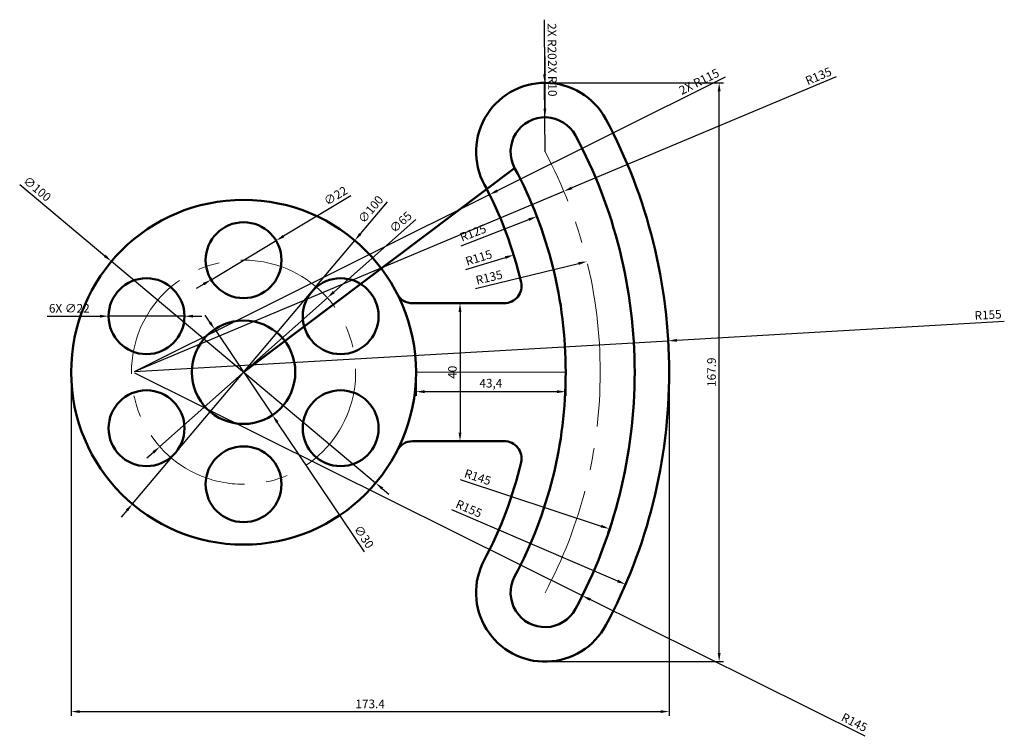
# Model space of a CAD drawing. Units: millimetres. Extents: x 3074 to 3359, y 1439 to 1647.
import ezdxf

# ---------------------------------------------------------------- set-up
doc = ezdxf.new("R2010")
doc.units = ezdxf.units.MM
doc.linetypes.add('CENTER', pattern=[50.8, 31.75, -6.35, 6.35, -6.35])
for name, color, linetype, lineweight in [('M-CNTR', 4, 'CENTER', 18), ('M-CONS', 8, 'Continuous', 13), ('M-DIMS', 2, 'Continuous', 25), ('M-OUTL', 7, 'Continuous', 50)]:
    doc.layers.add(name, color=color, linetype=linetype, lineweight=lineweight)
doc.styles.get("Standard").update_dxf_attribs({"font": 'arial.ttf'})
doc.dimstyles.new('ISO-25', dxfattribs={"dimtxt": 2.5, "dimasz": 2.5, "dimexe": 1.25, "dimexo": 0.625, "dimtad": 1, "dimtxsty": 'Standard', "dimcen": 2.5, "dimadec": 0, "dimazin": 0, "dimtfac": 1, "dimtmove": 0, "dimatfit": 3, "dimfxl": 1, "dimarcsym": 0})

# ---------------------------------------------------------------- blocks, each defined once
blk = doc.blocks.new('*D1')
at = {"layer": 'Defpoints', "color": 0, "transparency": 16777216}
for p in [(3188.62, 1545.09), (3232.02, 1545.09), (3188.62, 1539.45)]:
    blk.add_point(p, dxfattribs=at)
at = {"layer": 'M-DIMS', "color": 0, "lineweight": -2, "transparency": 16777216}
for p, q in [((3188.62, 1544.47), (3188.62, 1538.2)), ((3232.02, 1544.47), (3232.02, 1538.2)), ((3229.52, 1539.45), (3191.12, 1539.45))]:
    blk.add_line(p, q, dxfattribs=at)
at = {"layer": 'M-DIMS', "color": 0, "transparency": 16777216}
for points in [[(3191.12, 1539.87), (3191.12, 1539.03), (3188.62, 1539.45)], [(3229.52, 1539.87), (3229.52, 1539.03), (3232.02, 1539.45)]]:
    blk.add_solid(points, dxfattribs=at)
at = {"layer": 'M-DIMS', "color": 0, "transparency": 16777216, "insert": (3210.32, 1541.58), "char_height": 2.5, "attachment_point": 5}
blk.add_mtext('43,4', dxfattribs=at)
blk = doc.blocks.new('*D2')
at = {"layer": 'Defpoints', "color": 0, "transparency": 16777216}
for p in [(3223.66, 1590.27), (3107.02, 1545.32)]:
    blk.add_point(p, dxfattribs=at)
at = {"layer": 'M-DIMS', "color": 0, "lineweight": -2, "transparency": 16777216}
blk.add_line((3201.67, 1581.8), (3221.32, 1589.37), dxfattribs=at)
at = {"layer": 'M-DIMS', "color": 0, "transparency": 16777216}
blk.add_solid([(3221.17, 1589.76), (3221.47, 1588.98), (3223.66, 1590.27)], dxfattribs=at)
at = {"layer": 'M-DIMS', "color": 0, "transparency": 16777216, "insert": (3205.27, 1585.22), "char_height": 2.5, "attachment_point": 5, "rotation": 21.0776}
blk.add_mtext('R125', dxfattribs=at)
blk = doc.blocks.new('*D3')
at = {"layer": 'Defpoints', "color": 0, "transparency": 16777216}
for p in [(3216.94, 1579.11), (3107.02, 1545.32)]:
    blk.add_point(p, dxfattribs=at)
at = {"layer": 'M-DIMS', "color": 0, "lineweight": -2, "transparency": 16777216}
blk.add_line((3203.08, 1574.85), (3214.56, 1578.37), dxfattribs=at)
at = {"layer": 'M-DIMS', "color": 0, "transparency": 16777216}
blk.add_solid([(3214.43, 1578.77), (3214.68, 1577.97), (3216.94, 1579.11)], dxfattribs=at)
at = {"layer": 'M-DIMS', "color": 0, "transparency": 16777216, "insert": (3206.91, 1578.01), "char_height": 2.5, "attachment_point": 5, "rotation": 17.0867}
blk.add_mtext('R115', dxfattribs=at)
blk = doc.blocks.new('*D4')
at = {"layer": 'Defpoints', "color": 0, "transparency": 16777216}
for p in [(3238.2, 1577.23), (3107.02, 1545.32)]:
    blk.add_point(p, dxfattribs=at)
at = {"layer": 'M-DIMS', "color": 0, "lineweight": -2, "transparency": 16777216}
blk.add_line((3205.88, 1569.37), (3235.77, 1576.63), dxfattribs=at)
at = {"layer": 'M-DIMS', "color": 0, "transparency": 16777216}
blk.add_solid([(3235.67, 1577.04), (3235.87, 1576.23), (3238.2, 1577.23)], dxfattribs=at)
at = {"layer": 'M-DIMS', "color": 0, "transparency": 16777216, "insert": (3209.9, 1572.3), "char_height": 2.5, "attachment_point": 5, "rotation": 13.6714}
blk.add_mtext('R135', dxfattribs=at)
blk = doc.blocks.new('*D5')
at = {"layer": 'Defpoints', "color": 0, "transparency": 16777216}
for p in [(3107.02, 1545.32), (3244.65, 1499.68)]:
    blk.add_point(p, dxfattribs=at)
at = {"layer": 'M-DIMS', "color": 0, "lineweight": -2, "transparency": 16777216}
blk.add_line((3201.45, 1514), (3242.28, 1500.46), dxfattribs=at)
blk.add_arc((3107.02, 1545.32), 145, 341.1592, 359.6499, dxfattribs=at)
at = {"layer": 'M-DIMS', "color": 0, "transparency": 16777216}
blk.add_solid([(3242.41, 1500.86), (3242.15, 1500.07), (3244.65, 1499.68)], dxfattribs=at)
at = {"layer": 'M-DIMS', "color": 0, "transparency": 16777216, "insert": (3206.41, 1514.36), "char_height": 2.5, "attachment_point": 5, "rotation": 341.6531}
blk.add_mtext('R145', dxfattribs=at)
blk = doc.blocks.new('*D6')
at = {"layer": 'Defpoints', "color": 0, "transparency": 16777216}
for p in [(3107.02, 1544.87), (3249.38, 1483.55)]:
    blk.add_point(p, dxfattribs=at)
at = {"layer": 'M-DIMS', "color": 0, "lineweight": -2, "transparency": 16777216}
blk.add_line((3198.87, 1505.31), (3247.08, 1484.54), dxfattribs=at)
at = {"layer": 'M-DIMS', "color": 0, "transparency": 16777216}
blk.add_solid([(3247.24, 1484.92), (3246.91, 1484.15), (3249.38, 1483.55)], dxfattribs=at)
at = {"layer": 'M-DIMS', "color": 0, "transparency": 16777216, "insert": (3203.84, 1505.23), "char_height": 2.5, "attachment_point": 5, "rotation": 336.6959}
blk.add_mtext('R155', dxfattribs=at)
blk = doc.blocks.new('*D7')
at = {"layer": 'Defpoints', "color": 0, "transparency": 16777216}
for p in [(3170.86, 1583.31), (3106.38, 1506.87)]:
    blk.add_point(p, dxfattribs=at)
at = {"layer": 'M-DIMS', "color": 0, "lineweight": -2, "transparency": 16777216}
for p, q in [((3180.28, 1594.48), (3172.47, 1585.22)), ((3106.38, 1506.87), (3170.86, 1583.31)), ((3104.77, 1504.96), (3103.16, 1503.05))]:
    blk.add_line(p, q, dxfattribs=at)
at = {"layer": 'M-DIMS', "color": 0, "transparency": 16777216}
for points in [[(3172.15, 1585.49), (3172.79, 1584.96), (3170.86, 1583.31)], [(3104.45, 1505.23), (3105.09, 1504.69), (3106.38, 1506.87)]]:
    blk.add_solid(points, dxfattribs=at)
at = {"layer": 'M-DIMS', "color": 0, "transparency": 16777216, "insert": (3175.71, 1592.13), "char_height": 2.5, "attachment_point": 5, "rotation": 49.8536}
blk.add_mtext('∅100', dxfattribs=at)
blk = doc.blocks.new('*D8')
at = {"layer": 'Defpoints', "color": 0, "transparency": 16777216}
for p in [(3148.05, 1583.26), (3129.19, 1571.93)]:
    blk.add_point(p, dxfattribs=at)
at = {"layer": 'M-DIMS', "color": 0, "lineweight": -2, "transparency": 16777216}
for p, q in [((3169.71, 1596.27), (3150.19, 1584.55)), ((3129.19, 1571.93), (3148.05, 1583.26)), ((3127.05, 1570.64), (3124.91, 1569.35))]:
    blk.add_line(p, q, dxfattribs=at)
at = {"layer": 'M-DIMS', "color": 0, "transparency": 16777216}
for points in [[(3149.98, 1584.9), (3150.41, 1584.19), (3148.05, 1583.26)], [(3126.83, 1571), (3127.26, 1570.28), (3129.19, 1571.93)]]:
    blk.add_solid(points, dxfattribs=at)
at = {"layer": 'M-DIMS', "color": 0, "transparency": 16777216, "insert": (3165.47, 1596.02), "char_height": 2.5, "attachment_point": 5, "rotation": 30.9998}
blk.add_mtext('∅22', dxfattribs=at)
blk = doc.blocks.new('*D9')
at = {"layer": 'Defpoints', "color": 0, "transparency": 16777216}
for p in [(3162.91, 1566.68), (3114.33, 1523.5)]:
    blk.add_point(p, dxfattribs=at)
at = {"layer": 'M-DIMS', "color": 0, "lineweight": -2, "transparency": 16777216}
for p, q in [((3188.52, 1589.44), (3164.78, 1568.34)), ((3114.33, 1523.5), (3162.91, 1566.68)), ((3112.46, 1521.84), (3110.59, 1520.18))]:
    blk.add_line(p, q, dxfattribs=at)
at = {"layer": 'M-DIMS', "color": 0, "transparency": 16777216}
for points in [[(3164.5, 1568.66), (3165.06, 1568.03), (3162.91, 1566.68)], [(3112.18, 1522.15), (3112.74, 1521.53), (3114.33, 1523.5)]]:
    blk.add_solid(points, dxfattribs=at)
at = {"layer": 'M-DIMS', "color": 0, "transparency": 16777216, "insert": (3184.38, 1588.4), "char_height": 2.5, "attachment_point": 5, "rotation": 41.6293}
blk.add_mtext('∅65', dxfattribs=at)
blk = doc.blocks.new('*D10')
at = {"layer": 'Defpoints', "color": 0, "transparency": 16777216}
for p in [(3130.24, 1557.54), (3147, 1532.65)]:
    blk.add_point(p, dxfattribs=at)
at = {"layer": 'M-DIMS', "color": 0, "lineweight": -2, "transparency": 16777216}
for p, q in [((3128.85, 1559.61), (3127.45, 1561.68)), ((3130.24, 1557.54), (3147, 1532.65)), ((3173.73, 1492.95), (3148.4, 1530.58))]:
    blk.add_line(p, q, dxfattribs=at)
at = {"layer": 'M-DIMS', "color": 0, "transparency": 16777216}
for points in [[(3129.19, 1559.84), (3128.5, 1559.38), (3130.24, 1557.54)], [(3148.74, 1530.81), (3148.05, 1530.34), (3147, 1532.65)]]:
    blk.add_solid(points, dxfattribs=at)
at = {"layer": 'M-DIMS', "color": 0, "transparency": 16777216, "insert": (3173.26, 1497.18), "char_height": 2.5, "attachment_point": 5, "rotation": 303.9562}
blk.add_mtext('∅30', dxfattribs=at)
blk = doc.blocks.new('*D11')
at = {"layer": 'Defpoints', "color": 0, "transparency": 16777216}
for p in [(3200.9, 1565.09), (3200.9, 1525.09), (3201.38, 1525.09)]:
    blk.add_point(p, dxfattribs=at)
at = {"layer": 'M-DIMS', "color": 0, "lineweight": -2, "transparency": 16777216}
for p, q in [((3201.53, 1565.09), (3202.63, 1565.09)), ((3201.38, 1562.59), (3201.38, 1527.59)), ((3201.53, 1525.09), (3202.63, 1525.09))]:
    blk.add_line(p, q, dxfattribs=at)
at = {"layer": 'M-DIMS', "color": 0, "transparency": 16777216}
for points in [[(3200.96, 1562.59), (3201.8, 1562.59), (3201.38, 1565.09)], [(3200.96, 1527.59), (3201.8, 1527.59), (3201.38, 1525.09)]]:
    blk.add_solid(points, dxfattribs=at)
at = {"layer": 'M-DIMS', "color": 0, "transparency": 16777216, "insert": (3199.48, 1545.09), "char_height": 2.5, "attachment_point": 5, "rotation": 90}
blk.add_mtext('40', dxfattribs=at)
blk = doc.blocks.new('BOLT-HOLE-D22')
blk.add_circle((11, 11), 11)
blk = doc.blocks.new('*D13')
at = {"layer": 'Defpoints', "color": 0, "transparency": 16777216}
for p in [(3088.62, 1545.09), (3262.02, 1545.04), (3262.02, 1446.66)]:
    blk.add_point(p, dxfattribs=at)
at = {"layer": 'M-DIMS', "color": 0, "lineweight": -2, "transparency": 16777216}
for p, q in [((3088.62, 1544.47), (3088.62, 1445.41)), ((3262.02, 1544.41), (3262.02, 1445.41)), ((3091.12, 1446.66), (3259.52, 1446.66))]:
    blk.add_line(p, q, dxfattribs=at)
at = {"layer": 'M-DIMS', "color": 0, "transparency": 16777216}
for points in [[(3091.12, 1447.07), (3091.12, 1446.24), (3088.62, 1446.66)], [(3259.52, 1447.07), (3259.52, 1446.24), (3262.02, 1446.66)]]:
    blk.add_solid(points, dxfattribs=at)
at = {"layer": 'M-DIMS', "color": 0, "transparency": 16777216, "insert": (3175.32, 1448.56), "char_height": 2.5, "attachment_point": 5}
blk.add_mtext('173.4', dxfattribs=at)
blk = doc.blocks.new('*D14')
at = {"layer": 'Defpoints', "color": 0, "transparency": 16777216}
for p in [(3226.16, 1629.04), (3276.52, 1629.04), (3226.67, 1461.16)]:
    blk.add_point(p, dxfattribs=at)
at = {"layer": 'M-DIMS', "color": 0, "lineweight": -2, "transparency": 16777216}
for p, q in [((3226.78, 1629.04), (3277.77, 1629.04)), ((3276.52, 1463.66), (3276.52, 1626.54)), ((3227.3, 1461.16), (3277.77, 1461.16))]:
    blk.add_line(p, q, dxfattribs=at)
at = {"layer": 'M-DIMS', "color": 0, "transparency": 16777216}
for points in [[(3276.1, 1626.54), (3276.94, 1626.54), (3276.52, 1629.04)], [(3276.1, 1463.66), (3276.94, 1463.66), (3276.52, 1461.16)]]:
    blk.add_solid(points, dxfattribs=at)
at = {"layer": 'M-DIMS', "color": 0, "transparency": 16777216, "insert": (3274.62, 1545.1), "char_height": 2.5, "attachment_point": 5, "rotation": 90}
blk.add_mtext('167.9', dxfattribs=at)
blk = doc.blocks.new('*D15')
at = {"layer": 'Defpoints', "color": 0, "transparency": 16777216}
for p in [(3100.32, 1577.23), (3176.92, 1512.95)]:
    blk.add_point(p, dxfattribs=at)
at = {"layer": 'M-DIMS', "color": 0, "lineweight": -2, "transparency": 16777216}
for p, q in [((3073.7, 1599.56), (3098.4, 1578.84)), ((3176.92, 1512.95), (3100.32, 1577.23)), ((3178.84, 1511.35), (3180.75, 1509.74))]:
    blk.add_line(p, q, dxfattribs=at)
at = {"layer": 'M-DIMS', "color": 0, "transparency": 16777216}
for points in [[(3098.67, 1579.16), (3098.14, 1578.52), (3100.32, 1577.23)], [(3179.11, 1511.67), (3178.57, 1511.03), (3176.92, 1512.95)]]:
    blk.add_solid(points, dxfattribs=at)
at = {"layer": 'M-DIMS', "color": 0, "transparency": 16777216, "insert": (3078.6, 1598.03), "char_height": 2.5, "attachment_point": 5, "rotation": 319.9997}
blk.add_mtext('∅100', dxfattribs=at)
blk = doc.blocks.new('*D16')
at = {"layer": 'Defpoints', "color": 0, "transparency": 16777216}
for p in [(3099.47, 1561.34), (3121.47, 1561.34)]:
    blk.add_point(p, dxfattribs=at)
at = {"layer": 'M-DIMS', "color": 0, "lineweight": -2, "transparency": 16777216}
for p, q in [((3081.7, 1561.34), (3096.97, 1561.34)), ((3121.47, 1561.34), (3099.47, 1561.34)), ((3123.97, 1561.34), (3126.47, 1561.34))]:
    blk.add_line(p, q, dxfattribs=at)
at = {"layer": 'M-DIMS', "color": 0, "transparency": 16777216}
for points in [[(3096.97, 1561.76), (3096.97, 1560.93), (3099.47, 1561.34)], [(3123.97, 1561.76), (3123.97, 1560.93), (3121.47, 1561.34)]]:
    blk.add_solid(points, dxfattribs=at)
at = {"layer": 'M-DIMS', "color": 0, "transparency": 16777216, "insert": (3088.09, 1563.31), "char_height": 2.5, "attachment_point": 5, "rotation": 0.0006}
blk.add_mtext('6X ∅22', dxfattribs=at)
blk = doc.blocks.new('*D17')
at = {"layer": 'Defpoints', "color": 0, "transparency": 16777216}
for p in [(3209.94, 1596.62), (3107.02, 1545.32)]:
    blk.add_point(p, dxfattribs=at)
at = {"layer": 'M-DIMS', "color": 0, "lineweight": -2, "transparency": 16777216}
for p, q in [((3278.23, 1630.66), (3212.18, 1597.74)), ((3107.02, 1545.32), (3209.94, 1596.62))]:
    blk.add_line(p, q, dxfattribs=at)
at = {"layer": 'M-DIMS', "color": 0, "transparency": 16777216}
blk.add_solid([(3211.99, 1598.11), (3212.37, 1597.36), (3209.94, 1596.62)], dxfattribs=at)
at = {"layer": 'M-DIMS', "color": 0, "transparency": 16777216, "insert": (3270.85, 1629.11), "char_height": 2.5, "attachment_point": 5, "rotation": 26.4947}
blk.add_mtext('2X R115', dxfattribs=at)
blk = doc.blocks.new('*D18')
at = {"layer": 'Defpoints', "color": 0, "transparency": 16777216}
for p in [(3231.49, 1597.59), (3107.02, 1545.32)]:
    blk.add_point(p, dxfattribs=at)
at = {"layer": 'M-DIMS', "color": 0, "lineweight": -2, "transparency": 16777216}
for p, q in [((3310.41, 1630.73), (3233.8, 1598.56)), ((3107.02, 1545.32), (3231.49, 1597.59))]:
    blk.add_line(p, q, dxfattribs=at)
at = {"layer": 'M-DIMS', "color": 0, "transparency": 16777216}
blk.add_solid([(3233.63, 1598.94), (3233.96, 1598.17), (3231.49, 1597.59)], dxfattribs=at)
at = {"layer": 'M-DIMS', "color": 0, "transparency": 16777216, "insert": (3305.44, 1630.7), "char_height": 2.5, "attachment_point": 5, "rotation": 22.7791}
blk.add_mtext('R135', dxfattribs=at)
blk = doc.blocks.new('*D19')
at = {"layer": 'Defpoints', "color": 0, "transparency": 16777216}
for p in [(3107.02, 1544.87), (3236.84, 1480.28)]:
    blk.add_point(p, dxfattribs=at)
at = {"layer": 'M-DIMS', "color": 0, "lineweight": -2, "transparency": 16777216}
for p, q in [((3107.02, 1544.87), (3236.84, 1480.28)), ((3318.84, 1439.48), (3239.08, 1479.17))]:
    blk.add_line(p, q, dxfattribs=at)
at = {"layer": 'M-DIMS', "color": 0, "transparency": 16777216}
blk.add_solid([(3239.26, 1479.54), (3238.89, 1478.79), (3236.84, 1480.28)], dxfattribs=at)
at = {"layer": 'M-DIMS', "color": 0, "transparency": 16777216, "insert": (3315.58, 1443.23), "char_height": 2.5, "attachment_point": 5, "rotation": 333.5486}
blk.add_mtext('R145', dxfattribs=at)
blk = doc.blocks.new('*D20')
at = {"layer": 'Defpoints', "color": 0, "transparency": 16777216}
for p in [(3261.77, 1554.2), (3107.02, 1545.32)]:
    blk.add_point(p, dxfattribs=at)
at = {"layer": 'M-DIMS', "color": 0, "lineweight": -2, "transparency": 16777216}
for p, q in [((3359.2, 1559.79), (3264.26, 1554.34)), ((3107.02, 1545.32), (3261.77, 1554.2))]:
    blk.add_line(p, q, dxfattribs=at)
at = {"layer": 'M-DIMS', "color": 0, "transparency": 16777216}
blk.add_solid([(3264.24, 1554.76), (3264.29, 1553.93), (3261.77, 1554.2)], dxfattribs=at)
at = {"layer": 'M-DIMS', "color": 0, "transparency": 16777216, "insert": (3354.5, 1561.42), "char_height": 2.5, "attachment_point": 5, "rotation": 3.2843}
blk.add_mtext('R155', dxfattribs=at)
blk = doc.blocks.new('*D21')
at = {"layer": 'Defpoints', "color": 0, "transparency": 16777216}
for p in [(3225.9, 1629.04), (3226.03, 1609.04)]:
    blk.add_point(p, dxfattribs=at)
at = {"layer": 'M-DIMS', "color": 0, "lineweight": -2, "transparency": 16777216}
for p, q in [((3225.78, 1647.36), (3225.88, 1631.54)), ((3226.03, 1609.04), (3225.9, 1629.04))]:
    blk.add_line(p, q, dxfattribs=at)
at = {"layer": 'M-DIMS', "color": 0, "transparency": 16777216}
blk.add_solid([(3226.3, 1631.54), (3225.47, 1631.54), (3225.9, 1629.04)], dxfattribs=at)
at = {"layer": 'M-DIMS', "color": 0, "transparency": 16777216, "insert": (3227.72, 1641.05), "char_height": 2.5, "attachment_point": 5, "rotation": 270.3851}
blk.add_mtext('2X R20', dxfattribs=at)
blk = doc.blocks.new('*D22')
at = {"layer": 'Defpoints', "color": 0, "transparency": 16777216}
for p in [(3226, 1619.04), (3226.03, 1609.04)]:
    blk.add_point(p, dxfattribs=at)
at = {"layer": 'M-DIMS', "color": 0, "lineweight": -2, "transparency": 16777216}
for p, q in [((3225.94, 1636.67), (3225.99, 1621.54)), ((3226.03, 1609.04), (3226, 1619.04))]:
    blk.add_line(p, q, dxfattribs=at)
at = {"layer": 'M-DIMS', "color": 0, "transparency": 16777216}
blk.add_solid([(3226.41, 1621.54), (3225.57, 1621.54), (3226, 1619.04)], dxfattribs=at)
at = {"layer": 'M-DIMS', "color": 0, "transparency": 16777216, "insert": (3227.86, 1630.36), "char_height": 2.5, "attachment_point": 5, "rotation": 270.1978}
blk.add_mtext('2X R10', dxfattribs=at)

msp = doc.modelspace()

# ---------------------------------------------------------------- linework, layer by layer
at = {"layer": 'M-CNTR'}
msp.add_circle((3138.62, 1545.093), 32.5, dxfattribs=at)
for centre, start, end in [((3107.021, 1545.318), 359.89688, 28.16583), ((3107.021, 1544.868), 331.83417, 0.10312)]:
    msp.add_arc(centre, 135, start, end, dxfattribs=at)
at = {"layer": 'M-CONS'}
msp.add_line((3188.62, 1545.093), (3232.02, 1545.093), dxfattribs=at)
at = {"layer": 'M-OUTL'}
for points in [[(3262.02, 1545.039, 0.1239759), (3243.666, 1618.482, 1.0394281), (3209.185, 1598.267)], [(3252.02, 1545.057, 0.1239759), (3234.851, 1613.762, 1), (3217.219, 1604.321)], [(3138.62, 1545.093), (3217.219, 1604.321, -0.1239759), (3232.02, 1545.093, -0.1239759), (3217.219, 1485.865, 1), (3234.851, 1476.425, 0.1239759), (3252.02, 1545.129)], [(3183.157, 1567.82, 0.2818611), (3187.61, 1565.093), (3214.194, 1565.093, 0.4824302), (3219.066, 1571.219, 0.0661989), (3208.403, 1599.601)], [(3183.157, 1522.366, -0.2818611), (3187.61, 1525.093), (3214.194, 1525.093, -0.4824302), (3219.066, 1518.967, -0.0661989), (3208.403, 1490.585, 1), (3243.666, 1471.704, 0.1239759), (3262.02, 1545.147)]]:
    msp.add_lwpolyline(points, format="xyb", dxfattribs=at)
for radius in [50, 15]:
    msp.add_circle((3138.62, 1545.093), radius, dxfattribs=at)

# ---------------------------------------------------------------- block references
for p in [(3127.62, 1566.593), (3099.474, 1550.343), (3155.766, 1550.343), (3099.474, 1517.843), (3155.766, 1517.843), (3127.62, 1501.593)]:
    msp.add_blockref('BOLT-HOLE-D22', p, dxfattribs=at)

# ---------------------------------------------------------------- dimensions: what is measured, and where the dimension line sits
at = {"layer": 'M-DIMS'}
for center, mpoint, picture, middle in [((3226.035, 1609.041), (3225.9, 1629.041), '*D21', (3225.82, 1641.041)), ((3107.021, 1545.318), (3209.943, 1596.621), '*D17', (3271.696, 1627.403))]:
    dim = msp.add_radius_dim(center=center, mpoint=mpoint, text='2X <>', dimstyle='ISO-25', override={"dimdec": 0, "dimlfac": 1, "dimrnd": 0, "dimzin": 0, "dimdsep": 46, "dimlunit": 2}, dxfattribs=at)
    dim.commit()
    dim.dimension.update_dxf_attribs({"geometry": picture, "text_midpoint": middle, "dimtype": 164})
dim = msp.add_radius_dim(center=(3226.035, 1609.041), mpoint=(3226, 1619.041), text='2X <>', dimstyle='ISO-25', override={"dimdec": 0, "dimlfac": 1, "dimrnd": 0, "dimzin": 0, "dimdsep": 46, "dimlunit": 2}, dxfattribs=at)
dim.commit()
dim.dimension.update_dxf_attribs({"geometry": '*D22', "text_midpoint": (3227.863, 1630.363)})
for center, mpoint, override, picture, middle in [((3107.021, 1545.318), (3231.491, 1597.587), {"dimdec": 0, "dimlfac": 1, "dimrnd": 0, "dimzin": 0, "dimdsep": 46, "dimlunit": 2}, '*D18', (3306.174, 1628.949)), ((3107.021, 1545.318), (3223.657, 1590.272), {"dimclrd": 0, "dimclre": 0, "dimclrt": 0}, '*D2', (3205.958, 1583.451)), ((3107.021, 1545.318), (3216.945, 1579.107), {"dimclrd": 0, "dimclre": 0, "dimclrt": 0}, '*D3', (3207.471, 1576.195)), ((3107.021, 1545.318), (3238.196, 1577.226), {"dimclrd": 0, "dimclre": 0, "dimclrt": 0}, '*D4', (3210.345, 1570.451)), ((3107.021, 1545.318), (3261.766, 1554.198), {"dimdec": 0, "dimlfac": 1, "dimrnd": 0, "dimzin": 0, "dimdsep": 46, "dimlunit": 2}, '*D20', (3354.613, 1559.526)), ((3107.021, 1545.318), (3244.65, 1499.676), {"dimclrd": 0, "dimclre": 0, "dimclrt": 0}, '*D5', (3205.807, 1512.558)), ((3107.021, 1544.868), (3249.376, 1483.548), {"dimclrd": 0, "dimclre": 0, "dimclrt": 0}, '*D6', (3203.085, 1503.488)), ((3107.021, 1544.868), (3236.841, 1480.28), {"dimdec": 0, "dimlfac": 1, "dimrnd": 0, "dimzin": 0, "dimdsep": 46, "dimlunit": 2}, '*D19', (3314.733, 1441.526))]:
    dim = msp.add_radius_dim(center=center, mpoint=mpoint, dimstyle='ISO-25', override=override, dxfattribs=at)
    dim.commit()
    dim.dimension.update_dxf_attribs({"geometry": picture, "text_midpoint": middle, "dimtype": 164})
for base, p1, p2, override, picture, middle in [((3276.52, 1629.041), (3226.675, 1461.155), (3226.159, 1629.041), {"dimdec": 1, "dimlfac": 1, "dimrnd": 0, "dimzin": 0, "dimdsep": 46, "dimlunit": 2}, '*D14', (3274.619, 1545.098)), ((3201.379, 1525.093), (3200.902, 1565.093), (3200.902, 1525.093), {"dimclrd": 0, "dimclre": 0, "dimclrt": 0}, '*D11', (3199.478, 1545.093))]:
    dim = msp.add_linear_dim(base=base, p1=p1, p2=p2, angle=90, dimstyle='ISO-25', override=override, dxfattribs=at)
    dim.commit()
    dim.dimension.update_dxf_attribs({"geometry": picture, "text_midpoint": middle})
for p1, p2, override, picture, middle in [((3176.923, 1512.954), (3100.318, 1577.233), {"dimdec": 0, "dimlfac": 1, "dimrnd": 0, "dimzin": 0, "dimdsep": 46, "dimlunit": 2}, '*D15', (3077.337, 1596.516)), ((3129.192, 1571.928), (3148.049, 1583.259), {"dimclrd": 0, "dimclre": 0, "dimclrt": 0}, '*D8', (3166.482, 1594.334)), ((3106.383, 1506.873), (3170.858, 1583.313), {"dimclrd": 0, "dimclre": 0, "dimclrt": 0}, '*D7', (3177.221, 1590.857)), ((3114.328, 1523.503), (3162.913, 1566.683), {"dimclrd": 0, "dimclre": 0, "dimclrt": 0}, '*D9', (3185.691, 1586.927)), ((3130.242, 1557.535), (3146.999, 1532.651), {"dimclrd": 0, "dimclre": 0, "dimclrt": 0}, '*D10', (3171.625, 1496.082))]:
    dim = msp.add_diameter_dim_2p(p1=p1, p2=p2, dimstyle='ISO-25', override=override, dxfattribs=at)
    dim.commit()
    dim.dimension.update_dxf_attribs({"geometry": picture, "text_midpoint": middle, "dimtype": 163})
dim = msp.add_diameter_dim_2p(p1=(3121.475, 1561.343), p2=(3099.475, 1561.343), text='6X <>', dimstyle='ISO-25', override={"dimdec": 0, "dimlfac": 1, "dimrnd": 0, "dimzin": 0, "dimdsep": 46, "dimlunit": 2}, dxfattribs=at)
dim.commit()
dim.dimension.update_dxf_attribs({"geometry": '*D16', "text_midpoint": (3088.086, 1561.343), "dimtype": 163})
for base, p1, p2, override, picture, middle in [((3262.02, 1446.655), (3088.62, 1545.093), (3262.02, 1545.039), {"dimdec": 1, "dimlfac": 1, "dimrnd": 0, "dimzin": 0, "dimdsep": 46, "dimlunit": 2}, '*D13', (3175.32, 1448.557)), ((3188.62, 1539.45), (3232.02, 1545.093), (3188.62, 1545.093), {"dimclrd": 0, "dimclre": 0, "dimclrt": 0}, '*D1', (3210.32, 1541.577))]:
    dim = msp.add_linear_dim(base=base, p1=p1, p2=p2, dimstyle='ISO-25', override=override, dxfattribs=at)
    dim.commit()
    dim.dimension.update_dxf_attribs({"geometry": picture, "text_midpoint": middle})

doc.saveas('drawing.dxf')
